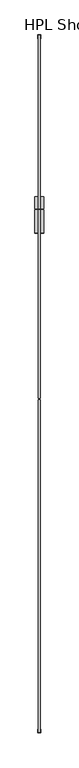
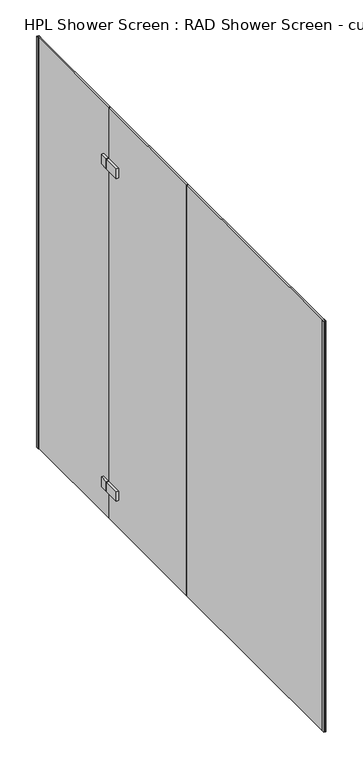
"""IFC4 building model written with IfcOpenShell, lengths in millimetres: flow terminal geometry, HPL Shower Screen : RAD Shower Screen - cut corner."""

from ifc_helpers import new_model, si_unit, frame, origin, origin_with_axes, place, context, project, spatial, polyline, outline, extrude, source, transform, mapped, element, save


def hpl_shower_screen_rad_shower_screen_cut_corner_ba801a97(model_context):
    return source(origin(), model_context, "Body", "SweptSolid", [
        extrude(outline(polyline([(18.1750129, 0.0), (18.1750129, -650.0), (11.8249871, -650.0), (11.8249871, 0.0), (18.1750129, 0.0)])), origin_with_axes(), (0.0, 0.0, 1.0), 2100.0),
        extrude(outline(polyline([(30.0, 0.0), (30.0, -80.0), (0.0, -80.0), (0.0, 0.0), (30.0, 0.0)])), frame((0.0, 0.0, 140.0), z_axis=(0.0, 0.0, 1.0), x_axis=(1.0, 0.0, 0.0)), (0.0, 0.0, 1.0), 50.0),
        extrude(outline(polyline([(30.0, 0.0), (30.0, -80.0), (0.0, -80.0), (0.0, 0.0), (30.0, 0.0)])), frame((0.0, 0.0, 1790.0), z_axis=(0.0, 0.0, 1.0), x_axis=(1.0, 0.0, 0.0)), (0.0, 0.0, 1.0), 50.0),
        extrude(outline(polyline([(11.8249871, 600.0), (18.1750129, 600.0), (18.1750129, 4.0), (11.8249871, 4.0), (11.8249871, 600.0)])), origin_with_axes(), (0.0, 0.0, 1.0), 2100.0),
        extrude(outline(polyline([(0.0, 44.0), (30.0, 44.0), (30.0, 4.0), (0.0, 4.0), (0.0, 44.0)])), frame((0.0, 0.0, 140.0), z_axis=(0.0, 0.0, 1.0), x_axis=(1.0, 0.0, 0.0)), (0.0, 0.0, 1.0), 50.0),
        extrude(outline(polyline([(0.0, 44.0), (30.0, 44.0), (30.0, 4.0), (0.0, 4.0), (0.0, 44.0)])), frame((0.0, 0.0, 1790.0), z_axis=(0.0, 0.0, 1.0), x_axis=(1.0, 0.0, 0.0)), (0.0, 0.0, 1.0), 50.0),
        extrude(outline(polyline([(11.8249871, -1800.0), (11.8249871, -655.0), (18.1750129, -655.0), (18.1750129, -1800.0), (11.8249871, -1800.0)])), origin_with_axes(), (0.0, 0.0, 1.0), 2100.0),
        extrude(outline(polyline([(11.8249871, 600.0), (11.8249871, 589.5), (9.8249871, 589.5), (9.8249871, 602.0), (20.1750129, 602.0), (20.1750129, 589.5), (18.1750129, 589.5), (18.1750129, 600.0), (11.8249871, 600.0)])), origin_with_axes(), (0.0, 0.0, 1.0), 2100.0),
        extrude(outline(polyline([(11.8249871, -1800.0), (18.1750129, -1800.0), (18.1750129, -1789.5), (20.1750129, -1789.5), (20.1750129, -1802.0), (9.8249871, -1802.0), (9.8249871, -1789.5), (11.8249871, -1789.5), (11.8249871, -1800.0)])), origin_with_axes(), (0.0, 0.0, 1.0), 2100.0),
    ])


if __name__ == "__main__":
    model = new_model("IFC4")
    model_context = context("Model", 3, world=origin())
    ifc_project = project(units=[si_unit("LENGTHUNIT", "METRE", prefix="MILLI")], contexts=[model_context])
    site = spatial("IfcSite", under=ifc_project)
    building = spatial("IfcBuilding", under=site)
    placement = place(None, origin())
    hpl_shower_screen_rad_shower_screen_cut_corner_shape = hpl_shower_screen_rad_shower_screen_cut_corner_ba801a97(model_context)
    element("IfcFlowTerminal", 1, ObjectType="HPL Shower Screen : RAD Shower Screen - cut corner", at=placement, inside=building, context=model_context, shape_type="MappedRepresentation", body=[
        mapped(hpl_shower_screen_rad_shower_screen_cut_corner_shape, transform((0.0, 0.0, 0.0), x_axis=(1.0, 0.0, 0.0), y_axis=(0.0, 1.0, 0.0), z_axis=(0.0, 0.0, 1.0))),
    ])
    save(model, "model.ifc")

# Revit data of these elements
# Type "HPL Shower Screen : RAD Shower Screen - cut corner"
#   URL = "http://www.matki.co.uk/"
#   Model = "EPW1150 BESPOKE - 'Eauzone Plus' - left hand recess"
#   Manufacturer = "MATKI"
#   Description = "Shower screen - chamfered fixed panel"
#   Fixed panel width [instance default] = 296 mm
#   End Panel Width [instance default] = 100 mm
#   Door Width = 650 mm
#   Offset = 0 mm
#   Height = 2100 mm
#   Door [instance default] = yes
#   Default Elevation = 0
# Element 1 (IfcFlowTerminal, "HPL Shower Screen : RAD Shower Screen - cut corner")
#   Fixed panel width = 596 mm
#   End Panel Width = 1145 mm
#   Materials on its faces: "Metal Joint", "Aluminum 5052", "Glass"
# Materials
#   "Metal Joint": colour RGB 247 247 247, transparency 0
#   "Aluminum 5052": class "Metal", colour RGB 120 120 120, transparency 0, Description = "Aluminum, strain hardened, magnesium alloy, marine", Cost = 0
#   "Glass": class "Glass", colour RGB 0 128 192, transparency 0.9, Description = "Soda Lime Glass", Cost = 0
